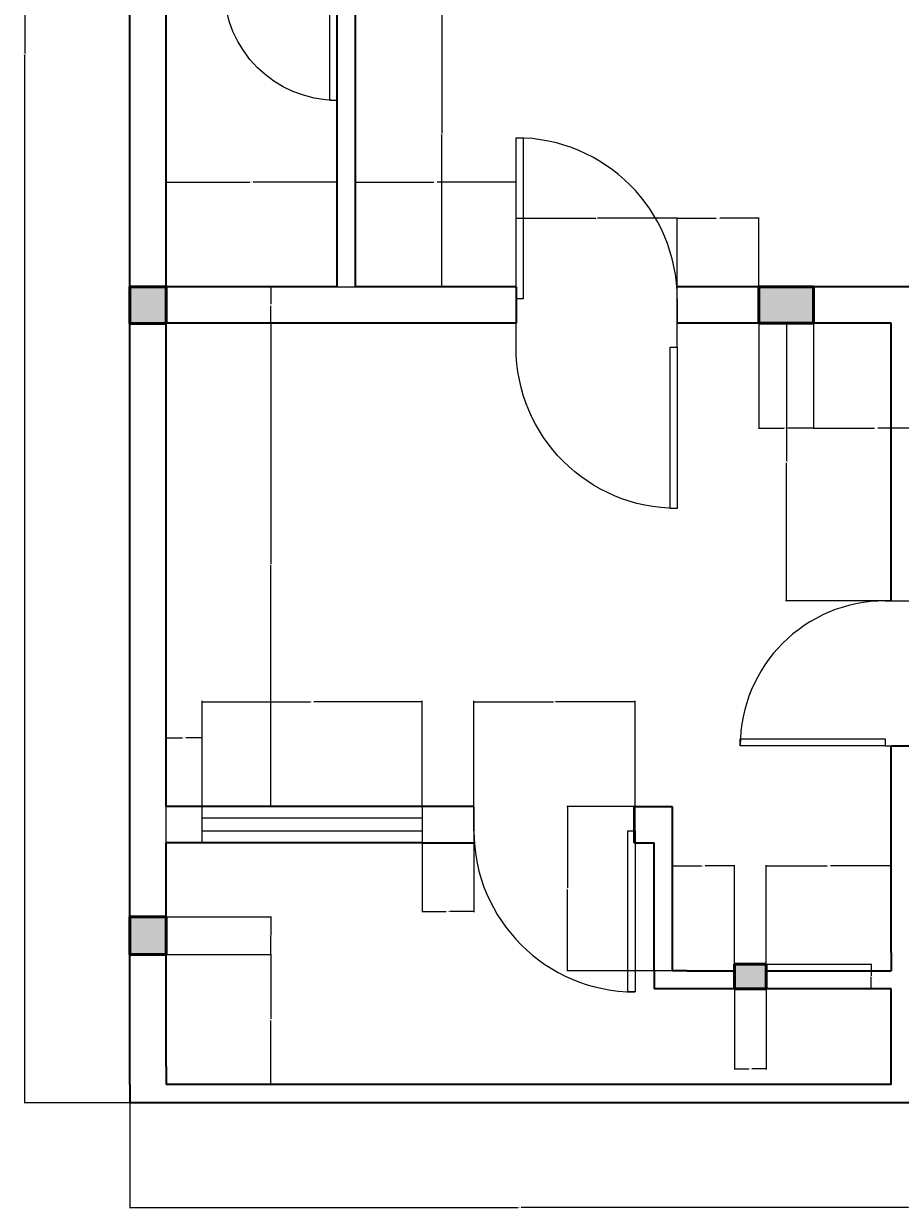
# Model space of a CAD drawing. Units: inches. Extents: x 229 to 651, y 108 to 681.
# Tile 1 of 4: x 229 to 447, y 108 to 402. Entities that reach past the tile are written whole.
import ezdxf

# ---------------------------------------------------------------- set-up
doc = ezdxf.new("R2010")
doc.units = ezdxf.units.IN
doc.header["$MEASUREMENT"] = 0
for name, color, linetype, lineweight in [('A-ANNO-DIMS', 2, 'Continuous', 18), ('A-COLS', 7, 'Continuous', 50), ('A-COLS-PATT', 5, 'Continuous', 13), ('A-DOOR', 3, 'Continuous', 25), ('A-GLAZ', 4, 'Continuous', 18), ('A-WALL', 7, 'Continuous', 35)]:
    doc.layers.add(name, color=color, linetype=linetype, lineweight=lineweight)
doc.styles.get("Standard").update_dxf_attribs({"font": 'arial.ttf'})
doc.dimstyles.get("Standard").update_dxf_attribs({"dimtxt": 0.18, "dimasz": 0.18, "dimexe": 0.18, "dimexo": 0.0625, "dimgap": 0.09, "dimtad": 0, "dimtih": 1, "dimtoh": 1, "dimdec": 4, "dimzin": 0, "dimdsep": 46, "dimtxsty": 'Standard', "dimcen": 0.09, "dimadec": 0, "dimazin": 0, "dimtfac": 1, "dimtdec": 4, "dimtofl": 0, "dimtmove": 0, "dimatfit": 3, "dimfxl": 1, "dimtolj": 1, "dimtzin": 0, "dimarcsym": 0})

# ---------------------------------------------------------------- blocks, each defined once
blk = doc.blocks.new('*U2')
for p, q in [((0, 0), (0, -6)), ((40, 0), (40, -6))]:
    blk.add_line(p, q)
blk.add_lwpolyline([(0, 0), (0, 40), (1.75, 40), (1.75, 0)], close=True)
blk.add_arc((0, 0), 40, 0, 90)
blk = doc.blocks.new('*U8')
for p, q in [((-40, 0), (-40, 6)), ((0, 0), (0, 6))]:
    blk.add_line(p, q)
blk.add_lwpolyline([(0, 0), (0, -40), (-1.75, -40), (-1.75, 0)], close=True)
blk.add_arc((0, 0), 40, 180, 270)
blk = doc.blocks.new('*U4')
for p, q in [((0, 0), (0, -6)), ((36, 0), (36, -6))]:
    blk.add_line(p, q)
blk.add_lwpolyline([(0, 0), (0, 36), (1.75, 36), (1.75, 0)], close=True)
blk.add_arc((0, 0), 36, 0, 90)
blk = doc.blocks.new('*U3')
for p, q in [((0, 0), (0, -6)), ((-40, 0), (-40, -6))]:
    blk.add_line(p, q)
blk.add_lwpolyline([(0, 0), (0, 40), (-1.75, 40), (-1.75, 0)], close=True)
blk.add_arc((0, 0), 40, 90, 180)
blk = doc.blocks.new('*U9')
for p, q in [((-28, 0), (-28, -6)), ((0, 0), (0, -6))]:
    blk.add_line(p, q)
blk.add_lwpolyline([(0, 0), (0, 28), (-1.75, 28), (-1.75, 0)], close=True)
blk.add_arc((0, 0), 28, 90, 180)
blk = doc.blocks.new('*D14')
at = {"layer": 'A-ANNO-DIMS', "color": 0, "lineweight": -2, "transparency": 16777216}
for p, q in [((255.68, 655.09), (229.53, 655.09)), ((229.71, 654.91), (229.71, 395.02)), ((229.71, 134.77), (229.71, 394.65)), ((255.68, 134.59), (229.53, 134.59))]:
    blk.add_line(p, q, dxfattribs=at)
at = {"layer": 'A-ANNO-DIMS', "color": 0, "transparency": 16777216}
for points in [[(229.68, 654.91), (229.74, 654.91), (229.71, 655.09)], [(229.68, 134.77), (229.74, 134.77), (229.71, 134.59)]]:
    blk.add_solid(points, dxfattribs=at)
at = {"layer": 'Defpoints', "color": 0, "transparency": 16777216}
for p in [(229.71, 655.09), (255.74, 655.09), (255.74, 134.59)]:
    blk.add_point(p, dxfattribs=at)
at = {"layer": 'A-ANNO-DIMS', "color": 0, "transparency": 16777216, "insert": (229.71, 394.84), "char_height": 0.18, "attachment_point": 5}
blk.add_mtext('\\A1;520.5', dxfattribs=at)
blk = doc.blocks.new('*D18')
at = {"layer": 'A-ANNO-DIMS', "color": 0, "lineweight": -2, "transparency": 16777216}
for p, q in [((264.81, 328.09), (290.95, 328.09)), ((290.77, 327.91), (290.77, 268.27)), ((290.77, 208.27), (290.77, 267.9)), ((264.81, 208.09), (290.95, 208.09))]:
    blk.add_line(p, q, dxfattribs=at)
at = {"layer": 'A-ANNO-DIMS', "color": 0, "transparency": 16777216}
for points in [[(290.74, 327.91), (290.8, 327.91), (290.77, 328.09)], [(290.74, 208.27), (290.8, 208.27), (290.77, 208.09)]]:
    blk.add_solid(points, dxfattribs=at)
at = {"layer": 'Defpoints', "color": 0, "transparency": 16777216}
for p in [(264.74, 328.09), (264.74, 208.09), (290.77, 208.09)]:
    blk.add_point(p, dxfattribs=at)
at = {"layer": 'A-ANNO-DIMS', "color": 0, "transparency": 16777216, "insert": (290.77, 268.09), "char_height": 0.18, "attachment_point": 5}
blk.add_mtext('\\A1;120', dxfattribs=at)
blk = doc.blocks.new('*D38')
at = {"layer": 'A-ANNO-DIMS', "color": 0, "lineweight": -2, "transparency": 16777216}
for p, q in [((264.74, 337.15), (264.74, 363.3)), ((264.92, 363.12), (285.57, 363.12)), ((306.97, 363.12), (286.33, 363.12)), ((307.15, 337.15), (307.15, 363.3))]:
    blk.add_line(p, q, dxfattribs=at)
at = {"layer": 'A-ANNO-DIMS', "color": 0, "transparency": 16777216}
for points in [[(264.92, 363.15), (264.92, 363.09), (264.74, 363.12)], [(306.97, 363.15), (306.97, 363.09), (307.15, 363.12)]]:
    blk.add_solid(points, dxfattribs=at)
at = {"layer": 'Defpoints', "color": 0, "transparency": 16777216}
for p in [(307.15, 363.12), (264.74, 337.09), (307.15, 337.09)]:
    blk.add_point(p, dxfattribs=at)
at = {"layer": 'A-ANNO-DIMS', "color": 0, "transparency": 16777216, "insert": (285.95, 363.12), "char_height": 0.18, "attachment_point": 5}
blk.add_mtext('\\A1;42.41', dxfattribs=at)
blk = doc.blocks.new('*D39')
at = {"layer": 'A-ANNO-DIMS', "color": 0, "lineweight": -2, "transparency": 16777216}
for p, q in [((307.21, 412.88), (333.36, 412.88)), ((333.18, 412.7), (333.18, 375.16)), ((333.18, 337.27), (333.18, 374.8)), ((307.21, 337.09), (333.36, 337.09))]:
    blk.add_line(p, q, dxfattribs=at)
at = {"layer": 'A-ANNO-DIMS', "color": 0, "transparency": 16777216}
for points in [[(333.15, 412.7), (333.21, 412.7), (333.18, 412.88)], [(333.15, 337.27), (333.21, 337.27), (333.18, 337.09)]]:
    blk.add_solid(points, dxfattribs=at)
at = {"layer": 'Defpoints', "color": 0, "transparency": 16777216}
for p in [(307.15, 412.88), (307.15, 337.09), (333.18, 337.09)]:
    blk.add_point(p, dxfattribs=at)
at = {"layer": 'A-ANNO-DIMS', "color": 0, "transparency": 16777216, "insert": (333.18, 374.98), "char_height": 0.18, "attachment_point": 5}
blk.add_mtext('\\A1;75.79', dxfattribs=at)
blk = doc.blocks.new('*D49')
at = {"layer": 'A-ANNO-DIMS', "color": 0, "lineweight": -2, "transparency": 16777216}
for p, q in [((311.65, 337.15), (311.65, 363.3)), ((311.83, 363.12), (331.24, 363.12)), ((351.44, 363.12), (332.03, 363.12)), ((351.62, 337.15), (351.62, 363.3))]:
    blk.add_line(p, q, dxfattribs=at)
at = {"layer": 'A-ANNO-DIMS', "color": 0, "transparency": 16777216}
for points in [[(311.83, 363.15), (311.83, 363.09), (311.65, 363.12)], [(351.44, 363.15), (351.44, 363.09), (351.62, 363.12)]]:
    blk.add_solid(points, dxfattribs=at)
at = {"layer": 'Defpoints', "color": 0, "transparency": 16777216}
for p in [(351.62, 363.12), (311.65, 337.09), (351.62, 337.09)]:
    blk.add_point(p, dxfattribs=at)
at = {"layer": 'A-ANNO-DIMS', "color": 0, "transparency": 16777216, "insert": (331.64, 363.12), "char_height": 0.18, "attachment_point": 5}
blk.add_mtext('\\A1;39.97', dxfattribs=at)
blk = doc.blocks.new('*D50')
at = {"layer": 'A-ANNO-DIMS', "color": 0, "lineweight": -2, "transparency": 16777216}
for p, q in [((351.62, 328.15), (351.62, 354.3)), ((351.8, 354.12), (371.4, 354.12)), ((391.44, 354.12), (371.85, 354.12)), ((391.62, 328.15), (391.62, 354.3))]:
    blk.add_line(p, q, dxfattribs=at)
at = {"layer": 'A-ANNO-DIMS', "color": 0, "transparency": 16777216}
for points in [[(351.8, 354.15), (351.8, 354.09), (351.62, 354.12)], [(391.44, 354.15), (391.44, 354.09), (391.62, 354.12)]]:
    blk.add_solid(points, dxfattribs=at)
at = {"layer": 'Defpoints', "color": 0, "transparency": 16777216}
for p in [(391.62, 354.12), (351.62, 328.09), (391.62, 328.09)]:
    blk.add_point(p, dxfattribs=at)
at = {"layer": 'A-ANNO-DIMS', "color": 0, "transparency": 16777216, "insert": (371.62, 354.12), "char_height": 0.18, "attachment_point": 5}
blk.add_mtext('\\A1;40', dxfattribs=at)
blk = doc.blocks.new('*D51')
at = {"layer": 'A-ANNO-DIMS', "color": 0, "lineweight": -2, "transparency": 16777216}
for p, q in [((391.62, 328.15), (391.62, 354.3)), ((391.8, 354.12), (401.27, 354.12)), ((411.66, 354.12), (402.2, 354.12)), ((411.84, 328.15), (411.84, 354.3))]:
    blk.add_line(p, q, dxfattribs=at)
at = {"layer": 'A-ANNO-DIMS', "color": 0, "transparency": 16777216}
for points in [[(391.8, 354.15), (391.8, 354.09), (391.62, 354.12)], [(411.66, 354.15), (411.66, 354.09), (411.84, 354.12)]]:
    blk.add_solid(points, dxfattribs=at)
at = {"layer": 'Defpoints', "color": 0, "transparency": 16777216}
for p in [(411.84, 354.12), (391.62, 328.09), (411.84, 328.09)]:
    blk.add_point(p, dxfattribs=at)
at = {"layer": 'A-ANNO-DIMS', "color": 0, "transparency": 16777216, "insert": (401.73, 354.12), "char_height": 0.18, "attachment_point": 5}
blk.add_mtext('\\A1;20.217', dxfattribs=at)
blk = doc.blocks.new('*D52')
at = {"layer": 'A-ANNO-DIMS', "color": 0, "lineweight": -2, "transparency": 16777216}
for p, q in [((411.84, 328.02), (411.84, 301.88)), ((425.43, 328.02), (425.43, 301.88)), ((412.02, 302.06), (418.18, 302.06)), ((425.25, 302.06), (419.09, 302.06))]:
    blk.add_line(p, q, dxfattribs=at)
at = {"layer": 'A-ANNO-DIMS', "color": 0, "transparency": 16777216}
for points in [[(412.02, 302.09), (412.02, 302.03), (411.84, 302.06)], [(425.25, 302.09), (425.25, 302.03), (425.43, 302.06)]]:
    blk.add_solid(points, dxfattribs=at)
at = {"layer": 'Defpoints', "color": 0, "transparency": 16777216}
for p in [(411.84, 328.09), (425.43, 328.09), (411.84, 302.06)]:
    blk.add_point(p, dxfattribs=at)
at = {"layer": 'A-ANNO-DIMS', "color": 0, "transparency": 16777216, "insert": (418.63, 302.06), "char_height": 0.18, "attachment_point": 5}
blk.add_mtext('\\A1;13.586', dxfattribs=at)
blk = doc.blocks.new('*D53')
at = {"layer": 'A-ANNO-DIMS', "color": 0, "lineweight": -2, "transparency": 16777216}
for p, q in [((425.43, 328.02), (425.43, 301.88)), ((456.56, 328.02), (456.56, 301.88)), ((425.61, 302.06), (440.6, 302.06)), ((456.38, 302.06), (441.38, 302.06))]:
    blk.add_line(p, q, dxfattribs=at)
at = {"layer": 'A-ANNO-DIMS', "color": 0, "transparency": 16777216}
for points in [[(425.61, 302.09), (425.61, 302.03), (425.43, 302.06)], [(456.38, 302.09), (456.38, 302.03), (456.56, 302.06)]]:
    blk.add_solid(points, dxfattribs=at)
at = {"layer": 'Defpoints', "color": 0, "transparency": 16777216}
for p in [(425.43, 328.09), (456.56, 328.09), (425.43, 302.06)]:
    blk.add_point(p, dxfattribs=at)
at = {"layer": 'A-ANNO-DIMS', "color": 0, "transparency": 16777216, "insert": (440.99, 302.06), "char_height": 0.18, "attachment_point": 5}
blk.add_mtext('\\A1;31.13', dxfattribs=at)
blk = doc.blocks.new('*D57')
at = {"layer": 'A-ANNO-DIMS', "color": 0, "lineweight": -2, "transparency": 16777216}
for p, q in [((255.74, 134.52), (255.74, 108.38)), ((449.24, 134.52), (449.24, 108.38)), ((255.92, 108.56), (352.11, 108.56)), ((449.06, 108.56), (352.88, 108.56))]:
    blk.add_line(p, q, dxfattribs=at)
at = {"layer": 'A-ANNO-DIMS', "color": 0, "transparency": 16777216}
for points in [[(255.92, 108.59), (255.92, 108.53), (255.74, 108.56)], [(449.06, 108.59), (449.06, 108.53), (449.24, 108.56)]]:
    blk.add_solid(points, dxfattribs=at)
at = {"layer": 'Defpoints', "color": 0, "transparency": 16777216}
for p in [(255.74, 134.59), (449.24, 134.59), (449.24, 108.56)]:
    blk.add_point(p, dxfattribs=at)
at = {"layer": 'A-ANNO-DIMS', "color": 0, "transparency": 16777216, "insert": (352.49, 108.56), "char_height": 0.18, "attachment_point": 5}
blk.add_mtext('\\A1;193.5', dxfattribs=at)
blk = doc.blocks.new('*D60')
at = {"layer": 'A-ANNO-DIMS', "color": 0, "lineweight": -2, "transparency": 16777216}
for p, q in [((444.68, 328.09), (418.53, 328.09)), ((418.71, 327.91), (418.71, 293.8)), ((418.71, 259.33), (418.71, 293.44)), ((444.68, 259.15), (418.53, 259.15))]:
    blk.add_line(p, q, dxfattribs=at)
at = {"layer": 'A-ANNO-DIMS', "color": 0, "transparency": 16777216}
for points in [[(418.68, 327.91), (418.74, 327.91), (418.71, 328.09)], [(418.68, 259.33), (418.74, 259.33), (418.71, 259.15)]]:
    blk.add_solid(points, dxfattribs=at)
at = {"layer": 'Defpoints', "color": 0, "transparency": 16777216}
for p in [(418.71, 328.09), (444.74, 328.09), (444.74, 259.15)]:
    blk.add_point(p, dxfattribs=at)
at = {"layer": 'A-ANNO-DIMS', "color": 0, "transparency": 16777216, "insert": (418.71, 293.62), "char_height": 0.18, "attachment_point": 5}
blk.add_mtext('\\A1;68.93', dxfattribs=at)
blk = doc.blocks.new('*D61')
at = {"layer": 'A-ANNO-DIMS', "color": 0, "lineweight": -2, "transparency": 16777216}
for p, q in [((273.72, 208.15), (273.72, 234.3)), ((273.9, 234.12), (300.61, 234.12)), ((328.11, 234.12), (301.4, 234.12)), ((328.29, 208.15), (328.29, 234.3))]:
    blk.add_line(p, q, dxfattribs=at)
at = {"layer": 'A-ANNO-DIMS', "color": 0, "transparency": 16777216}
for points in [[(273.9, 234.15), (273.9, 234.09), (273.72, 234.12)], [(328.11, 234.15), (328.11, 234.09), (328.29, 234.12)]]:
    blk.add_solid(points, dxfattribs=at)
at = {"layer": 'Defpoints', "color": 0, "transparency": 16777216}
for p in [(328.29, 234.12), (273.72, 208.09), (328.29, 208.09)]:
    blk.add_point(p, dxfattribs=at)
at = {"layer": 'A-ANNO-DIMS', "color": 0, "transparency": 16777216, "insert": (301, 234.12), "char_height": 0.18, "attachment_point": 5}
blk.add_mtext('\\A1;54.57', dxfattribs=at)
blk = doc.blocks.new('*D62')
at = {"layer": 'A-ANNO-DIMS', "color": 0, "lineweight": -2, "transparency": 16777216}
for p, q in [((328.29, 208.02), (328.29, 181.88)), ((341.15, 208.02), (341.15, 181.88)), ((328.47, 182.06), (334.26, 182.06)), ((340.97, 182.06), (335.17, 182.06))]:
    blk.add_line(p, q, dxfattribs=at)
at = {"layer": 'A-ANNO-DIMS', "color": 0, "transparency": 16777216}
for points in [[(328.47, 182.09), (328.47, 182.03), (328.29, 182.06)], [(340.97, 182.09), (340.97, 182.03), (341.15, 182.06)]]:
    blk.add_solid(points, dxfattribs=at)
at = {"layer": 'Defpoints', "color": 0, "transparency": 16777216}
for p in [(328.29, 208.09), (341.15, 208.09), (328.29, 182.06)]:
    blk.add_point(p, dxfattribs=at)
at = {"layer": 'A-ANNO-DIMS', "color": 0, "transparency": 16777216, "insert": (334.72, 182.06), "char_height": 0.18, "attachment_point": 5}
blk.add_mtext('\\A1;12.865', dxfattribs=at)
blk = doc.blocks.new('*D63')
at = {"layer": 'A-ANNO-DIMS', "color": 0, "lineweight": -2, "transparency": 16777216}
for p, q in [((341.15, 208.15), (341.15, 234.3)), ((341.33, 234.12), (360.93, 234.12)), ((380.97, 234.12), (361.37, 234.12)), ((381.15, 208.15), (381.15, 234.3))]:
    blk.add_line(p, q, dxfattribs=at)
at = {"layer": 'A-ANNO-DIMS', "color": 0, "transparency": 16777216}
for points in [[(341.33, 234.15), (341.33, 234.09), (341.15, 234.12)], [(380.97, 234.15), (380.97, 234.09), (381.15, 234.12)]]:
    blk.add_solid(points, dxfattribs=at)
at = {"layer": 'Defpoints', "color": 0, "transparency": 16777216}
for p in [(381.15, 234.12), (341.15, 208.09), (381.15, 208.09)]:
    blk.add_point(p, dxfattribs=at)
at = {"layer": 'A-ANNO-DIMS', "color": 0, "transparency": 16777216, "insert": (361.15, 234.12), "char_height": 0.18, "attachment_point": 5}
blk.add_mtext('\\A1;40', dxfattribs=at)
blk = doc.blocks.new('*D64')
at = {"layer": 'A-ANNO-DIMS', "color": 0, "lineweight": -2, "transparency": 16777216}
for p, q in [((413.72, 167.4), (413.72, 193.55)), ((413.9, 193.37), (428.84, 193.37)), ((444.56, 193.37), (429.63, 193.37)), ((444.74, 167.4), (444.74, 193.55))]:
    blk.add_line(p, q, dxfattribs=at)
at = {"layer": 'A-ANNO-DIMS', "color": 0, "transparency": 16777216}
for points in [[(413.9, 193.4), (413.9, 193.34), (413.72, 193.37)], [(444.56, 193.4), (444.56, 193.34), (444.74, 193.37)]]:
    blk.add_solid(points, dxfattribs=at)
at = {"layer": 'Defpoints', "color": 0, "transparency": 16777216}
for p in [(444.74, 193.37), (413.72, 167.34), (444.74, 167.34)]:
    blk.add_point(p, dxfattribs=at)
at = {"layer": 'A-ANNO-DIMS', "color": 0, "transparency": 16777216, "insert": (429.23, 193.37), "char_height": 0.18, "attachment_point": 5}
blk.add_mtext('\\A1;31.02', dxfattribs=at)
blk = doc.blocks.new('*D65')
at = {"layer": 'A-ANNO-DIMS', "color": 0, "lineweight": -2, "transparency": 16777216}
for p, q in [((390.34, 208.09), (364.2, 208.09)), ((364.38, 207.91), (364.38, 187.9)), ((364.38, 167.52), (364.38, 187.53)), ((390.34, 167.34), (364.2, 167.34))]:
    blk.add_line(p, q, dxfattribs=at)
at = {"layer": 'A-ANNO-DIMS', "color": 0, "transparency": 16777216}
for points in [[(364.35, 207.91), (364.41, 207.91), (364.38, 208.09)], [(364.35, 167.52), (364.41, 167.52), (364.38, 167.34)]]:
    blk.add_solid(points, dxfattribs=at)
at = {"layer": 'Defpoints', "color": 0, "transparency": 16777216}
for p in [(364.38, 208.09), (390.41, 208.09), (390.41, 167.34)]:
    blk.add_point(p, dxfattribs=at)
at = {"layer": 'A-ANNO-DIMS', "color": 0, "transparency": 16777216, "insert": (364.38, 187.71), "char_height": 0.18, "attachment_point": 5}
blk.add_mtext('\\A1;40.75', dxfattribs=at)
blk = doc.blocks.new('*D66')
at = {"layer": 'A-ANNO-DIMS', "color": 0, "lineweight": -2, "transparency": 16777216}
for p, q in [((264.74, 199.15), (264.74, 225.3)), ((264.92, 225.12), (268.84, 225.12)), ((273.54, 225.12), (269.62, 225.12)), ((273.72, 199.15), (273.72, 225.3))]:
    blk.add_line(p, q, dxfattribs=at)
at = {"layer": 'A-ANNO-DIMS', "color": 0, "transparency": 16777216}
for points in [[(264.92, 225.15), (264.92, 225.09), (264.74, 225.12)], [(273.54, 225.15), (273.54, 225.09), (273.72, 225.12)]]:
    blk.add_solid(points, dxfattribs=at)
at = {"layer": 'Defpoints', "color": 0, "transparency": 16777216}
for p in [(273.72, 225.12), (264.74, 199.09), (273.72, 199.09)]:
    blk.add_point(p, dxfattribs=at)
at = {"layer": 'A-ANNO-DIMS', "color": 0, "transparency": 16777216, "insert": (269.23, 225.12), "char_height": 0.18, "attachment_point": 5}
blk.add_mtext('\\A1;8.972', dxfattribs=at)
blk = doc.blocks.new('*D67')
at = {"layer": 'A-ANNO-DIMS', "color": 0, "lineweight": -2, "transparency": 16777216}
for p, q in [((264.81, 337.09), (290.95, 337.09)), ((290.77, 336.91), (290.77, 332.77)), ((290.77, 328.27), (290.77, 332.4)), ((264.81, 328.09), (290.95, 328.09))]:
    blk.add_line(p, q, dxfattribs=at)
at = {"layer": 'A-ANNO-DIMS', "color": 0, "transparency": 16777216}
for points in [[(290.74, 336.91), (290.8, 336.91), (290.77, 337.09)], [(290.74, 328.27), (290.8, 328.27), (290.77, 328.09)]]:
    blk.add_solid(points, dxfattribs=at)
at = {"layer": 'Defpoints', "color": 0, "transparency": 16777216}
for p in [(264.74, 337.09), (264.74, 328.09), (290.77, 328.09)]:
    blk.add_point(p, dxfattribs=at)
at = {"layer": 'A-ANNO-DIMS', "color": 0, "transparency": 16777216, "insert": (290.77, 332.59), "char_height": 0.18, "attachment_point": 5}
blk.add_mtext('\\A1;9', dxfattribs=at)
blk = doc.blocks.new('*D68')
at = {"layer": 'A-ANNO-DIMS', "color": 0, "lineweight": -2, "transparency": 16777216}
for p, q in [((264.81, 180.69), (290.95, 180.69)), ((290.77, 180.51), (290.77, 176.2)), ((290.77, 171.52), (290.77, 175.83)), ((264.81, 171.34), (290.95, 171.34))]:
    blk.add_line(p, q, dxfattribs=at)
at = {"layer": 'A-ANNO-DIMS', "color": 0, "transparency": 16777216}
for points in [[(290.74, 180.51), (290.8, 180.51), (290.77, 180.69)], [(290.74, 171.52), (290.8, 171.52), (290.77, 171.34)]]:
    blk.add_solid(points, dxfattribs=at)
at = {"layer": 'Defpoints', "color": 0, "transparency": 16777216}
for p in [(264.74, 180.69), (264.74, 171.34), (290.77, 171.34)]:
    blk.add_point(p, dxfattribs=at)
at = {"layer": 'A-ANNO-DIMS', "color": 0, "transparency": 16777216, "insert": (290.77, 176.01), "char_height": 0.18, "attachment_point": 5}
blk.add_mtext('\\A1;9.355', dxfattribs=at)
blk = doc.blocks.new('*D69')
at = {"layer": 'A-ANNO-DIMS', "color": 0, "lineweight": -2, "transparency": 16777216}
for p, q in [((264.81, 171.34), (290.95, 171.34)), ((290.77, 171.16), (290.77, 155.39)), ((290.77, 139.27), (290.77, 155.03)), ((264.81, 139.09), (290.95, 139.09))]:
    blk.add_line(p, q, dxfattribs=at)
at = {"layer": 'A-ANNO-DIMS', "color": 0, "transparency": 16777216}
for points in [[(290.74, 171.16), (290.8, 171.16), (290.77, 171.34)], [(290.74, 139.27), (290.8, 139.27), (290.77, 139.09)]]:
    blk.add_solid(points, dxfattribs=at)
at = {"layer": 'Defpoints', "color": 0, "transparency": 16777216}
for p in [(264.74, 171.34), (264.74, 139.09), (290.77, 139.09)]:
    blk.add_point(p, dxfattribs=at)
at = {"layer": 'A-ANNO-DIMS', "color": 0, "transparency": 16777216, "insert": (290.77, 155.21), "char_height": 0.18, "attachment_point": 5}
blk.add_mtext('\\A1;32.25', dxfattribs=at)
blk = doc.blocks.new('*D75')
at = {"layer": 'A-ANNO-DIMS', "color": 0, "lineweight": -2, "transparency": 16777216}
for p, q in [((390.41, 167.4), (390.41, 193.55)), ((390.59, 193.37), (397.67, 193.37)), ((405.66, 193.37), (398.58, 193.37)), ((405.84, 167.4), (405.84, 193.55))]:
    blk.add_line(p, q, dxfattribs=at)
at = {"layer": 'A-ANNO-DIMS', "color": 0, "transparency": 16777216}
for points in [[(390.59, 193.4), (390.59, 193.34), (390.41, 193.37)], [(405.66, 193.4), (405.66, 193.34), (405.84, 193.37)]]:
    blk.add_solid(points, dxfattribs=at)
at = {"layer": 'Defpoints', "color": 0, "transparency": 16777216}
for p in [(405.84, 193.37), (390.41, 167.34), (405.84, 167.34)]:
    blk.add_point(p, dxfattribs=at)
at = {"layer": 'A-ANNO-DIMS', "color": 0, "transparency": 16777216, "insert": (398.12, 193.37), "char_height": 0.18, "attachment_point": 5}
blk.add_mtext('\\A1;15.437', dxfattribs=at)
blk = doc.blocks.new('*D76')
at = {"layer": 'A-ANNO-DIMS', "color": 0, "lineweight": -2, "transparency": 16777216}
for p, q in [((405.84, 168.94), (405.84, 142.8)), ((413.72, 168.94), (413.72, 142.8)), ((406.02, 142.98), (409.39, 142.98)), ((413.54, 142.98), (410.18, 142.98))]:
    blk.add_line(p, q, dxfattribs=at)
at = {"layer": 'A-ANNO-DIMS', "color": 0, "transparency": 16777216}
for points in [[(406.02, 143.01), (406.02, 142.95), (405.84, 142.98)], [(413.54, 143.01), (413.54, 142.95), (413.72, 142.98)]]:
    blk.add_solid(points, dxfattribs=at)
at = {"layer": 'Defpoints', "color": 0, "transparency": 16777216}
for p in [(405.84, 169.01), (413.72, 169.01), (405.84, 142.98)]:
    blk.add_point(p, dxfattribs=at)
at = {"layer": 'A-ANNO-DIMS', "color": 0, "transparency": 16777216, "insert": (409.78, 142.98), "char_height": 0.18, "attachment_point": 5}
blk.add_mtext('\\A1;7.882', dxfattribs=at)
blk = doc.blocks.new('*D77')
at = {"layer": 'A-ANNO-DIMS', "color": 0, "lineweight": -2, "transparency": 16777216}
for p, q in [((413.79, 169.01), (439.93, 169.01)), ((439.75, 168.83), (439.75, 166.1)), ((439.75, 163.02), (439.75, 165.74)), ((413.79, 162.84), (439.93, 162.84))]:
    blk.add_line(p, q, dxfattribs=at)
at = {"layer": 'A-ANNO-DIMS', "color": 0, "transparency": 16777216}
for points in [[(439.72, 168.83), (439.78, 168.83), (439.75, 169.01)], [(439.72, 163.02), (439.78, 163.02), (439.75, 162.84)]]:
    blk.add_solid(points, dxfattribs=at)
at = {"layer": 'Defpoints', "color": 0, "transparency": 16777216}
for p in [(413.72, 169.01), (413.72, 162.84), (439.75, 162.84)]:
    blk.add_point(p, dxfattribs=at)
at = {"layer": 'A-ANNO-DIMS', "color": 0, "transparency": 16777216, "insert": (439.75, 165.92), "char_height": 0.18, "attachment_point": 5}
blk.add_mtext('\\A1;6.165', dxfattribs=at)

msp = doc.modelspace()

# ---------------------------------------------------------------- hatches: boundary and pattern name
at = {"layer": 'A-COLS-PATT'}
h = msp.add_hatch(color=256, dxfattribs=at)
h.dxf.hatch_style = 1
h.paths.add_polyline_path([(264.7698, 655.0869), (255.744, 655.0869), (255.744, 646.0869), (264.7698, 646.0869)])
h.paths.add_polyline_path([(428.5355, 655.0869), (414.8518, 655.0869), (414.8518, 646.0869), (428.5355, 646.0869)])
h.paths.add_polyline_path([(579.744, 655.0869), (568.5366, 655.0869), (568.5366, 646.0869), (570.744, 646.0869), (579.744, 646.0869)])
h.paths.add_polyline_path([(579.744, 468.8158), (570.744, 468.8158), (570.744, 457.0869), (579.744, 457.0869)])
h.paths.add_polyline_path([(422.244, 467.874), (416.0718, 467.874), (416.0718, 457.0869), (422.244, 457.0869)])
h.paths.add_polyline_path([(264.744, 465.8018), (255.744, 465.8018), (255.744, 453.3882), (264.744, 453.3882), (264.744, 457.0869)])
h.paths.add_polyline_path([(264.744, 337.0869), (255.744, 337.0869), (255.744, 328.0161), (264.744, 328.0161)])
h.paths.add_polyline_path([(425.426, 337.0869), (411.84, 337.0869), (411.84, 328.0869), (425.426, 328.0869)])
h.paths.add_polyline_path([(579.744, 337.0869), (570.744, 337.0869), (570.744, 328.0869), (579.744, 328.0869)])
h.paths.add_polyline_path([(579.744, 188.4262), (570.744, 188.4262), (570.744, 178.0508), (579.744, 178.0508)])
h.paths.add_polyline_path([(413.7248, 169.0053), (405.843, 169.0053), (405.843, 162.8404), (413.7248, 162.8404)])
h.paths.add_polyline_path([(264.744, 180.6917), (255.744, 180.6917), (255.744, 171.3369), (264.744, 171.3369)])

# ---------------------------------------------------------------- linework, layer by layer
at = {"layer": 'A-COLS'}
for p, q in [((264.744, 337.0869), (255.744, 337.0869)), ((255.744, 337.0869), (255.744, 328.0161)), ((264.744, 328.0869), (264.744, 337.0869)), ((425.426, 337.0869), (411.84, 337.0869)), ((411.84, 337.0869), (411.84, 328.0869)), ((425.426, 328.0869), (425.426, 337.0869)), ((255.744, 328.0161), (264.744, 328.0161)), ((411.84, 328.0869), (425.426, 328.0869)), ((255.744, 180.6917), (264.744, 180.6917)), ((255.744, 171.3369), (255.744, 180.6917)), ((264.744, 180.6917), (264.744, 171.3369)), ((264.744, 171.3369), (255.744, 171.3369)), ((405.843, 162.8404), (405.843, 169.0053)), ((405.843, 169.0053), (413.7248, 169.0053)), ((413.7248, 169.0053), (413.7248, 162.8404)), ((413.7248, 162.8404), (405.843, 162.8404))]:
    msp.add_line(p, q, dxfattribs=at)
at = {"layer": 'A-GLAZ'}
for p, q in [((273.7163, 199.0869), (273.7163, 208.0869)), ((273.7163, 208.0869), (319.1697, 208.0869)), ((328.2865, 208.0869), (328.2865, 199.0869)), ((273.7163, 205.3277), (328.2865, 205.3277)), ((328.2865, 202.0216), (273.7163, 202.0216)), ((284.0052, 199.0869), (328.2865, 199.0869)), ((319.1697, 199.0869), (328.2865, 199.0869))]:
    msp.add_line(p, q, dxfattribs=at)
at = {"layer": 'A-WALL'}
for p, q in [((255.744, 139.0869), (255.744, 655.0869)), ((264.744, 337.0869), (264.744, 457.0869)), ((311.6505, 457.0869), (311.6505, 337.0869)), ((307.1505, 417.1791), (307.1505, 337.0869)), ((307.1505, 337.0869), (264.744, 337.0869)), ((351.6231, 337.0869), (311.6505, 337.0869)), ((351.6231, 337.0869), (351.6231, 328.0869)), ((449.244, 337.0869), (391.5105, 337.0869)), ((264.744, 208.0869), (264.744, 328.0869)), ((351.6231, 328.0869), (264.744, 328.0869)), ((444.744, 328.0869), (391.6231, 328.0869)), ((444.744, 259.1543), (444.744, 328.0869)), ((444.744, 208.0869), (444.744, 223.1543)), ((444.744, 223.1543), (449.244, 223.1543)), ((341.1511, 208.0869), (264.744, 208.0869)), ((380.9058, 208.0869), (385.9062, 208.0869)), ((380.9058, 199.0869), (380.9058, 208.0869)), ((385.9062, 208.0869), (390.4062, 208.0869)), ((390.4062, 208.0869), (390.4062, 171.8404)), ((444.744, 171.8404), (444.744, 208.0869)), ((264.744, 143.5869), (264.744, 199.0869)), ((328.2865, 199.0869), (264.744, 199.0869)), ((328.2865, 199.0869), (341.2637, 199.0869)), ((380.9058, 199.0869), (385.9062, 199.0869)), ((385.9062, 167.3404), (385.9062, 199.0869)), ((390.4062, 171.8404), (390.4062, 167.3404)), ((444.744, 171.8404), (444.744, 167.3404)), ((385.9062, 167.3404), (385.9062, 162.8404)), ((394.103, 167.3404), (390.4062, 167.3404)), ((394.103, 167.3404), (405.843, 167.3404)), ((413.7248, 167.3404), (444.744, 167.3404)), ((389.603, 162.8404), (385.9062, 162.8404)), ((394.103, 162.8404), (389.603, 162.8404)), ((444.744, 162.8404), (394.103, 162.8404)), ((444.744, 139.0869), (444.744, 162.8404)), ((264.744, 143.5869), (264.744, 139.0869)), ((255.744, 139.0869), (255.744, 134.5869)), ((268.4408, 139.0869), (264.744, 139.0869)), ((444.744, 139.0869), (268.4408, 139.0869)), ((259.4408, 134.5869), (255.744, 134.5869)), ((268.4408, 134.5869), (259.4408, 134.5869)), ((449.244, 134.5869), (268.4408, 134.5869))]:
    msp.add_line(p, q, dxfattribs=at)

# ---------------------------------------------------------------- block references
at = {"layer": 'A-DOOR', "xscale": -1, "rotation": 180}
for name, p in [('*U9', (307.1505, 411.3792)), ('*U3', (391.6231, 322.0869))]:
    msp.add_blockref(name, p, dxfattribs=at)
at = {"layer": 'A-DOOR'}
for name, p in [('*U2', (351.6231, 334.0869)), ('*U8', (381.1511, 202.0869))]:
    msp.add_blockref(name, p, dxfattribs=at)
at = {"layer": 'A-DOOR', "rotation": 90}
msp.add_blockref('*U4', (443.244, 223.1543), dxfattribs=at)

# ---------------------------------------------------------------- dimensions: what is measured, and where the dimension line sits
at = {"layer": 'A-ANNO-DIMS'}
for base, p1, p2, angle, override, picture, middle in [((229.714, 655.0869), (255.744, 134.5869), (255.744, 655.0869), 90, {"dimdec": 1, "dimlfac": 1, "dimrnd": 0, "dimzin": 0, "dimdsep": 46, "dimlunit": 2}, '*D14', (229.714, 394.8369)), ((333.1805, 337.0869), (307.1505, 412.8792), (307.1505, 337.0869), 270, {"dimdec": 2, "dimlfac": 1, "dimrnd": 0, "dimzin": 0, "dimdsep": 46, "dimlunit": 2}, '*D39', (333.1805, 374.983)), ((290.774, 328.0869), (264.744, 337.0869), (264.744, 328.0869), 270, {"dimdec": 0, "dimlfac": 1, "dimrnd": 0, "dimzin": 0, "dimdsep": 46, "dimlunit": 2}, '*D67', (290.774, 332.5869)), ((290.774, 208.0869), (264.744, 328.0869), (264.744, 208.0869), 270, {"dimdec": 0, "dimlfac": 1, "dimrnd": 0, "dimzin": 0, "dimdsep": 46, "dimlunit": 2}, '*D18', (290.774, 268.0869)), ((411.84, 302.0569), (425.426, 328.0869), (411.84, 328.0869), 180, {"dimdec": 3, "dimlfac": 1, "dimrnd": 0, "dimzin": 0, "dimdsep": 46, "dimlunit": 2}, '*D52', (418.633, 302.0569)), ((418.714, 328.0869), (444.744, 259.1543), (444.744, 328.0869), 90, {"dimdec": 2, "dimlfac": 1, "dimrnd": 0, "dimzin": 0, "dimdsep": 46, "dimlunit": 2}, '*D60', (418.714, 293.6206)), ((425.426, 302.0569), (456.556, 328.0869), (425.426, 328.0869), 180, {"dimdec": 2, "dimlfac": 1, "dimrnd": 0, "dimzin": 0, "dimdsep": 46, "dimlunit": 2}, '*D53', (440.991, 302.0569)), ((328.2865, 182.0569), (341.1511, 208.0869), (328.2865, 208.0869), 180, {"dimdec": 3, "dimlfac": 1, "dimrnd": 0, "dimzin": 0, "dimdsep": 46, "dimlunit": 2}, '*D62', (334.7188, 182.0569)), ((364.3762, 208.0869), (390.4062, 167.3404), (390.4062, 208.0869), 90, {"dimdec": 2, "dimlfac": 1, "dimrnd": 0, "dimzin": 0, "dimdsep": 46, "dimlunit": 2}, '*D65', (364.3762, 187.7136)), ((405.843, 193.3704), (390.4062, 167.3404), (405.843, 167.3404), 0, {"dimdec": 3, "dimlfac": 1, "dimrnd": 0, "dimzin": 0, "dimdsep": 46, "dimlunit": 2}, '*D75', (398.1246, 193.3704)), ((290.774, 171.3369), (264.744, 180.6917), (264.744, 171.3369), 270, {"dimdec": 3, "dimlfac": 1, "dimrnd": 0, "dimzin": 0, "dimdsep": 46, "dimlunit": 2}, '*D68', (290.774, 176.0143)), ((290.774, 139.0869), (264.744, 171.3369), (264.744, 139.0869), 270, {"dimdec": 2, "dimlfac": 1, "dimrnd": 0, "dimzin": 0, "dimdsep": 46, "dimlunit": 2}, '*D69', (290.774, 155.2119)), ((405.843, 142.9753), (413.7248, 169.0053), (405.843, 169.0053), 180, {"dimdec": 3, "dimlfac": 1, "dimrnd": 0, "dimzin": 0, "dimdsep": 46, "dimlunit": 2}, '*D76', (409.7839, 142.9753)), ((439.7548, 162.8404), (413.7248, 169.0053), (413.7248, 162.8404), 270, {"dimdec": 3, "dimlfac": 1, "dimrnd": 0, "dimzin": 0, "dimdsep": 46, "dimlunit": 2}, '*D77', (439.7548, 165.9228))]:
    dim = msp.add_linear_dim(base=base, p1=p1, p2=p2, angle=angle, dimstyle='Standard', override=override, dxfattribs=at)
    dim.commit()
    dim.dimension.update_dxf_attribs({"geometry": picture, "text_midpoint": middle})
for base, p1, p2, override, picture, middle in [((307.1505, 363.1169), (264.744, 337.0869), (307.1505, 337.0869), {"dimdec": 2, "dimlfac": 1, "dimrnd": 0, "dimzin": 0, "dimdsep": 46, "dimlunit": 2}, '*D38', (285.9473, 363.1169)), ((351.6231, 363.1169), (311.6505, 337.0869), (351.6231, 337.0869), {"dimdec": 2, "dimlfac": 1, "dimrnd": 0, "dimzin": 0, "dimdsep": 46, "dimlunit": 2}, '*D49', (331.6368, 363.1169)), ((391.6231, 354.1169), (351.6231, 328.0869), (391.6231, 328.0869), {"dimdec": 0, "dimlfac": 1, "dimrnd": 0, "dimzin": 0, "dimdsep": 46, "dimlunit": 2}, '*D50', (371.6231, 354.1169)), ((411.84, 354.1169), (391.6231, 328.0869), (411.84, 328.0869), {"dimdec": 3, "dimlfac": 1, "dimrnd": 0, "dimzin": 0, "dimdsep": 46, "dimlunit": 2}, '*D51', (401.7316, 354.1169)), ((328.2865, 234.1169), (273.7163, 208.0869), (328.2865, 208.0869), {"dimdec": 2, "dimlfac": 1, "dimrnd": 0, "dimzin": 0, "dimdsep": 46, "dimlunit": 2}, '*D61', (301.0014, 234.1169)), ((381.1511, 234.1169), (341.1511, 208.0869), (381.1511, 208.0869), {"dimdec": 0, "dimlfac": 1, "dimrnd": 0, "dimzin": 0, "dimdsep": 46, "dimlunit": 2}, '*D63', (361.1511, 234.1169)), ((273.7163, 225.1169), (264.744, 199.0869), (273.7163, 199.0869), {"dimdec": 3, "dimlfac": 1, "dimrnd": 0, "dimzin": 0, "dimdsep": 46, "dimlunit": 2}, '*D66', (269.2302, 225.1169)), ((444.744, 193.3704), (413.7248, 167.3404), (444.744, 167.3404), {"dimdec": 2, "dimlfac": 1, "dimrnd": 0, "dimzin": 0, "dimdsep": 46, "dimlunit": 2}, '*D64', (429.2344, 193.3704)), ((449.244, 108.5569), (255.744, 134.5869), (449.244, 134.5869), {"dimdec": 1, "dimlfac": 1, "dimrnd": 0, "dimzin": 0, "dimdsep": 46, "dimlunit": 2}, '*D57', (352.494, 108.5569))]:
    dim = msp.add_linear_dim(base=base, p1=p1, p2=p2, dimstyle='Standard', override=override, dxfattribs=at)
    dim.commit()
    dim.dimension.update_dxf_attribs({"geometry": picture, "text_midpoint": middle})

doc.saveas('drawing.dxf')
